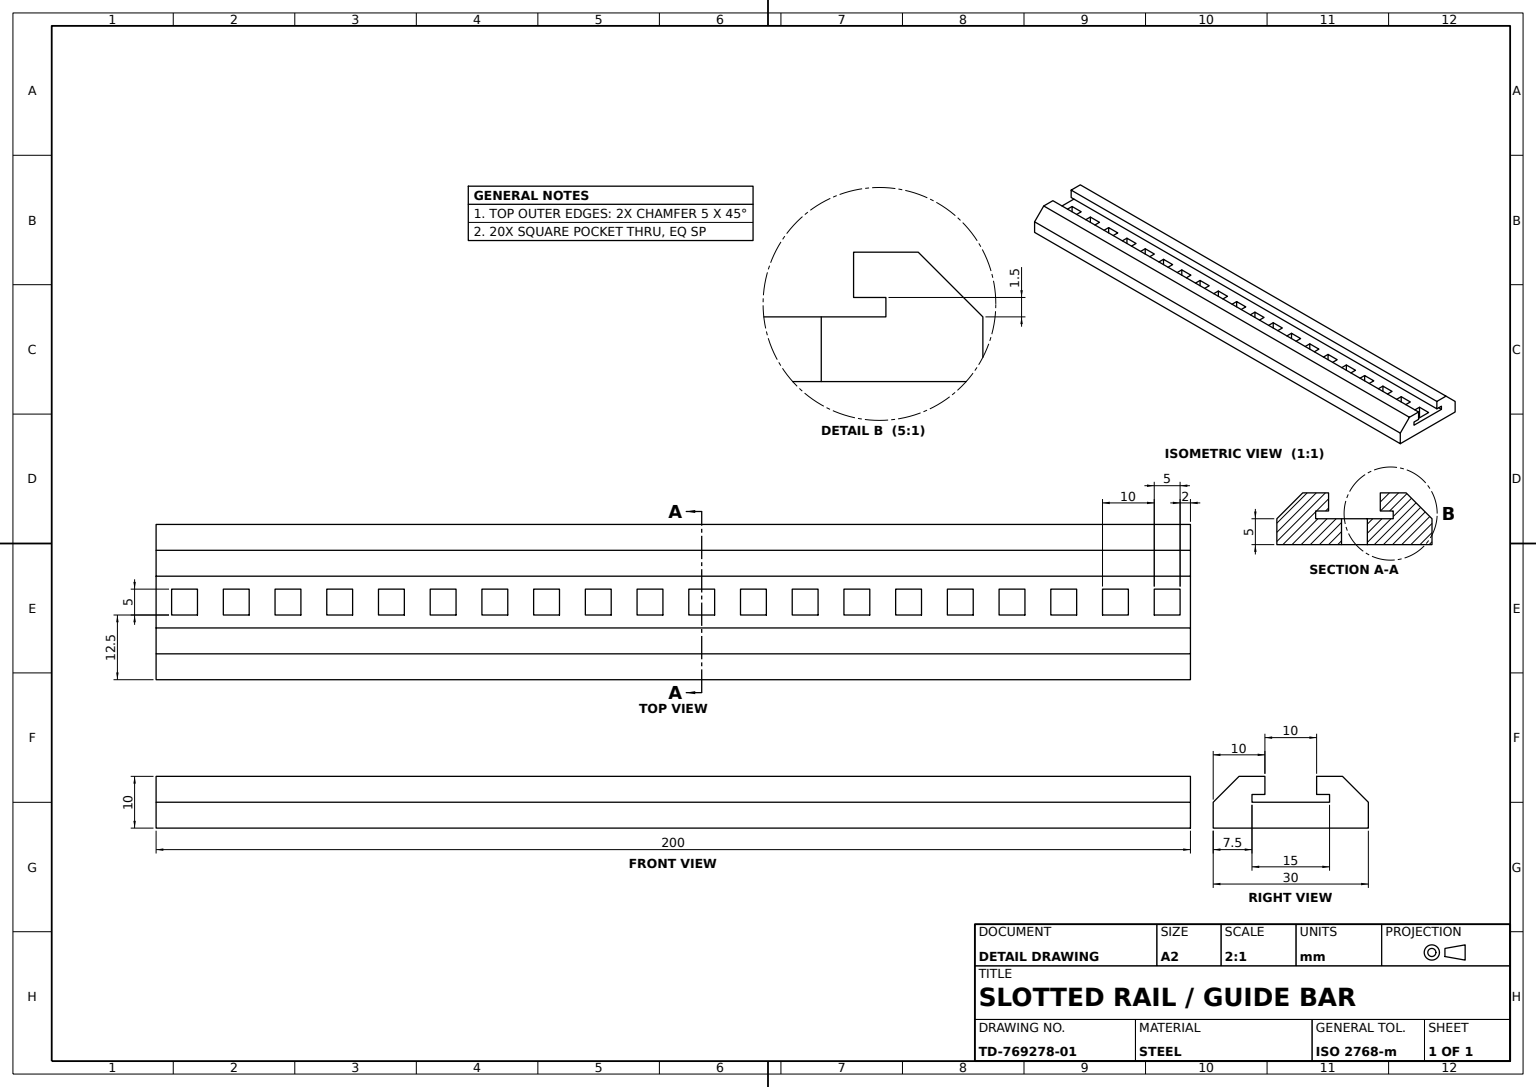
SolidWorks part; units mm, degrees
material "Plain Carbon Steel"
ref_plane "Front Plane" through (0, 0, 0) normal (0, 0, 1) x (1, 0, 0)
ref_plane "Top Plane" through (0, 0, 0) normal (0, 1, 0) x (1, 0, 0)
ref_plane "Right Plane" through (0, 0, 0) normal (1, 0, 0) x (0, 0, -1)
sketch "Track Profile Sketch" plane through (0, 0, 0) normal (0, 0, 1) x (1, 0, 0)
  line L1 (-15, 5) -> (15, 5)
  line L2 (-15, 5) -> (-15, -5)
  line L3 (-15, -5) -> (15, -5)
  line L4 (15, 5) -> (15, -5)
  line L5 (-15, 5) -> (15, -5) construction
  line L6 (-15, -5) -> (15, 5) construction
  point P0 (0, 0)
  dimension "D1" = 30
  dimension "D2" = 10
extrude "Track Body 200mm" add sketch "Track Profile Sketch" along normal mid plane 200
chamfer "Edge Chamfer 5mm" distance 5 angle 45 2 edges at (-15, 5, 0) (15, 5, 0)
sketch "Guide Groove Sketch" plane through (0, 5, 0) normal (0, 1, 0) x (1, 0, 0)
  line L0 (10, 100) -> (-10, 100) construction
  line L1 (-5, 100) -> (5, 100)
  line L2 (-5, 100) -> (-5, -100)
  line L3 (-5, -100) -> (5, -100)
  line L4 (5, 100) -> (5, -100)
  line L5 (10, -100) -> (-10, -100) construction
  line L6 (15, 100) -> (15, -100) construction
  line L7 (-15, -100) -> (-15, 100) construction
  dimension "D1" = 10
  dimension "D2" = 10
extrude "Guide Groove 10x5" cut sketch "Guide Groove Sketch" against normal blind 5
sketch "End Notch Sketch" plane through (0, 0, 100) normal (0, 0, 1) x (1, 0, 0)
  line L0 (-15, -5) -> (15, -5) construction
  line L1 (-7.5, 1.5) -> (7.5, 1.5)
  line L2 (-7.5, 1.5) -> (-7.5, 0)
  line L3 (-7.5, 0) -> (7.5, 0)
  line L4 (7.5, 1.5) -> (7.5, 0)
  dimension "D1" = 15
  dimension "D2" = 5
  dimension "D3" = 1.5
  dimension "D4" = 7.5
extrude "End Notch Cut" cut sketch "End Notch Sketch" against normal up to next
sketch "Rack Pocket Sketch" plane through (0, 0, 0) normal (0, 1, 0) x (1, 0, 0)
  line L0 (7.5, 100) -> (-7.5, 100) construction
  line L1 (-2.5, 98) -> (2.5, 98)
  line L2 (-2.5, 98) -> (-2.5, 93)
  line L3 (-2.5, 93) -> (2.5, 93)
  line L4 (2.5, 98) -> (2.5, 93)
  line L5 (-2.5, 98) -> (2.5, 93) construction
  line L6 (-2.5, 93) -> (2.5, 98) construction
  point P0 (0, 95.5)
  dimension "D1" = 5
  dimension "D2" = 5
  dimension "D3" = 2
extrude "Rack Pocket Cut" cut sketch "Rack Pocket Sketch" against normal up to next
pattern_linear "Rack Pocket Pattern 20x10mm" count 20 spacing 10 along (0, 0, 1) of "Rack Pocket Cut"
